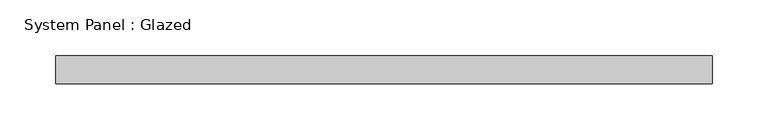
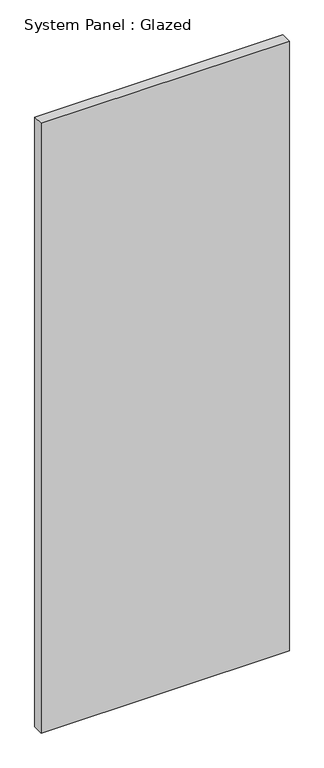
"""IFC4 building model written with IfcOpenShell, lengths in millimetres: plate geometry, System Panel : Glazed."""

from ifc_helpers import new_model, si_unit, origin, origin_with_axes, place, context, project, spatial, polyline, outline, extrude, source, transform, mapped, element, save


def system_panel_glazed_978b3bbc(model_context):
    return source(origin(), model_context, "Body", "SweptSolid", [
        extrude(outline(polyline([(295.275, 19.05), (-295.275, 19.05), (-295.275, 44.45), (295.275, 44.45), (295.275, 19.05)])), origin_with_axes(), (0.0, 0.0, 1.0), 1532.4287133),
    ])


if __name__ == "__main__":
    model = new_model("IFC4")
    model_context = context("Model", 3, world=origin())
    ifc_project = project(units=[si_unit("LENGTHUNIT", "METRE", prefix="MILLI")], contexts=[model_context])
    site = spatial("IfcSite", under=ifc_project)
    building = spatial("IfcBuilding", under=site)
    placement = place(None, origin())
    system_panel_glazed_shape = system_panel_glazed_978b3bbc(model_context)
    element("IfcPlate", 1, ObjectType="System Panel : Glazed", at=placement, inside=building, context=model_context, shape_type="MappedRepresentation", body=[
        mapped(system_panel_glazed_shape, transform((0.0, 0.0, 0.0), x_axis=(1.0, 0.0, 0.0), y_axis=(0.0, 1.0, 0.0), z_axis=(0.0, 0.0, 1.0))),
    ])
    save(model, "model.ifc")

# Revit data of these elements
# Type "System Panel : Glazed"
#   Construction Type Id = "GSP4R"
#   Analytic Construction = "1/8 in Pilkington single glazing"
#   Visual Light Transmittance = 0.9
#   Solar Heat Gain Coefficient = 0.86
#   Heat Transfer Coefficient (U) = 1.18115 BTU/(h·ft²·°F)
#   Define Thermal Properties by = 1
# Element 1 (IfcPlate, "System Panel : Glazed")
#   Materials on its faces: "Glass"
# Materials
#   "Glass": class "Glass", colour RGB 0 128 192, transparency 0.75, Description = "Soda Lime Glass", Cost = 0
